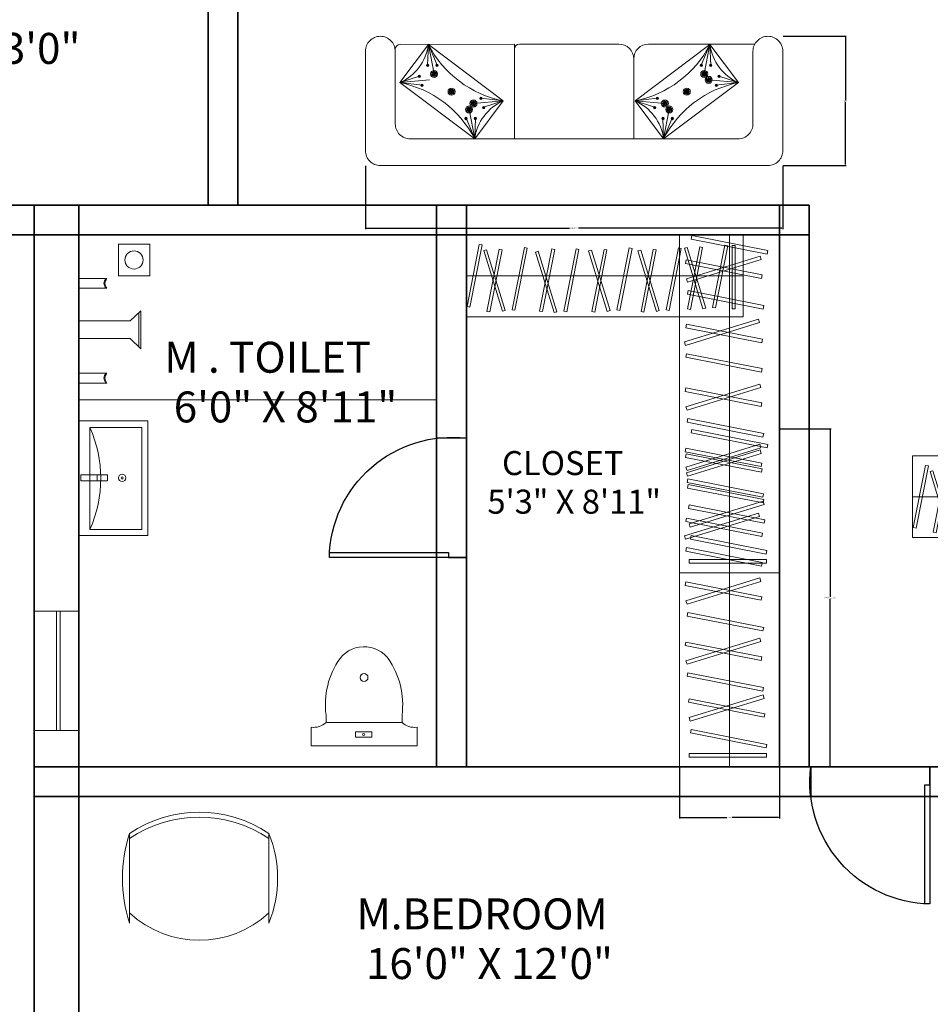
# Model space of a CAD drawing. Units: inches. Extents: x -61 to 1599, y -1316 to 257.
# Tile 18 of 204: x 76 to 259, y -1105 to -907. Entities that reach past the tile are written whole.
import ezdxf

# ---------------------------------------------------------------- set-up
doc = ezdxf.new("R2010")
doc.units = ezdxf.units.IN
doc.header["$MEASUREMENT"] = 0
doc.linetypes.add('ACAD_ISO02W100', pattern=[15, 12, -3])
for name, color, linetype, lineweight in [('A-ANNO-DIMS', 2, 'Continuous', 18), ('A-AREA-IDEN', 1, 'Continuous', 18), ('A-FLOR-CASE', 8, 'Continuous', 18), ('A-FLOR-FIXT', 8, 'Continuous', 18), ('A-WALL-JAMB', 4, 'ACAD_ISO02W100', 25), ('DOORS', 2, 'Continuous', 25), ('FURNITURE', 83, 'Continuous', 18), ('WALLS', 4, 'Continuous', 35), ('WINDOWS', 220, 'Continuous', 18)]:
    doc.layers.add(name, color=color, linetype=linetype, lineweight=lineweight)
doc.layers.add('FUR', color=83, linetype='Continuous')
doc.styles.get("Standard").update_dxf_attribs({"font": 'arial.ttf'})
doc.dimstyles.get("Standard").update_dxf_attribs({"dimtxt": 0.18, "dimasz": 0.18, "dimexe": 0.18, "dimexo": 0.0625, "dimgap": 0.09, "dimtad": 0, "dimtih": 1, "dimtoh": 1, "dimdec": 0, "dimzin": 0, "dimdsep": 46, "dimlunit": 3, "dimtxsty": 'Standard', "dimcen": 0.09, "dimadec": 0, "dimazin": 0, "dimtfac": 1, "dimtdec": 0, "dimtofl": 0, "dimtmove": 0, "dimatfit": 3, "dimfxl": 1, "dimtolj": 1, "dimtzin": 0, "dimarcsym": 0})

# ---------------------------------------------------------------- blocks, each defined once
blk = doc.blocks.new('DOOR-SWING-24')
blk.add_line((0, 0), (0, 3.6))
blk.add_lwpolyline([(0, 0), (0, -24), (1.05, -24), (1.05, 0)], close=True)
blk.add_arc((-0.44, 0.62), 24.62, 271.0259, 6.9559)
blk = doc.blocks.new('WIN-24IN')
for p, q in [((0, 4.5), (0, 9)), ((0, 9), (0, 0)), ((24, 9), (24, 0)), ((0, 5.19), (24, 5.19)), ((0, 4.5), (24, 4.5))]:
    blk.add_line(p, q)
blk = doc.blocks.new('WC-FLOOR-MOUNT')
for p, q in [((3.02, 4.69), (3.02, 6.17)), ((18.31, 4.69), (18.31, 6.17)), ((3.02, 4.69), (18.31, 4.69)), ((0, 0), (0, 3.75)), ((21.33, 0), (21.33, 3.75)), ((0, 0), (21.33, 0))]:
    blk.add_line(p, q)
blk.add_lwpolyline([(12.24, 1.73), (8.96, 1.73), (8.96, 2.81), (12.24, 2.81)], close=True)
for centre, radius in [((10.67, 13.73), 0.792), ((10.6, 2.27), 0.208)]:
    blk.add_circle(centre, radius)
for centre, radius, start, end in [((10.67, 13.73), 6.18, 27.6844, 141.4697), ((19.05, 8.26), 16.17, 144.824, 187.4232), ((2.28, 8.26), 16.17, 352.5768, 35.176), ((0.56, 7.25), 3.55, 260.8586, 313.6993), ((20.77, 7.25), 3.55, 226.3007, 279.1414)]:
    blk.add_arc(centre, radius, start, end)
blk = doc.blocks.new('LAVATORY-WALL-2')
blk.add_line((3.67, 10.96), (3.67, 12.19))
for points in [[(0, 23.07), (13.87, 23.07), (13.87, 0), (0, 0)], [(12.66, 21.73), (12.66, 1.19), (2.2, 1.19), (2.2, 21.73)], [(5.78, 12.19), (5.78, 10.96), (0.4, 10.96), (0.4, 12.19)]]:
    blk.add_lwpolyline(points, close=True)
for radius in [0.74, 0.233]:
    blk.add_circle((8.7, 11.57), radius)
blk.add_arc((-20.86, 11.46), 25.25, 335.9939, 24.0061)
blk = doc.blocks.new('SHOWER-FITTINGS-3')
for p, q in [((0, 21.03), (5.62, 21.03)), ((0, 19.05), (5.62, 19.05)), ((10.34, 12.49), (12.46, 14.54)), ((12.05, 14.15), (12.05, 7.29)), ((12.46, 14.54), (12.46, 6.9)), ((0, 12.49), (10.34, 12.49)), ((0, 8.95), (10.34, 8.95)), ((10.34, 8.95), (12.46, 6.9)), ((0, 1.97), (5.62, 1.97)), ((0, 0), (5.62, 0))]:
    blk.add_line(p, q)
blk.add_lwpolyline([(14.24, 21.57), (7.95, 21.57), (7.95, 27.94), (14.24, 27.94)], close=True)
blk.add_circle((11.09, 24.76), 1.83)
for points in [[(5.44, 21.03), (5.24, 20.71), (4.83, 20.05), (5.23, 19.39), (5.44, 19.05)], [(5.62, 21.03), (5.42, 20.71), (5.02, 20.05), (5.42, 19.39), (5.62, 19.05)], [(5.44, 1.97), (5.24, 1.65), (4.83, 1), (5.23, 0.34), (5.44, 0)], [(5.62, 1.97), (5.42, 1.65), (5.02, 1), (5.42, 0.34), (5.62, 0)]]:
    blk.add_open_spline(points, degree=3, knots=[0, 0, 0, 0, 1.043806, 2.132489, 2.132489, 2.132489, 2.132489])
blk = doc.blocks.new('BEDROOM-CHAIR')
for p, q in [((1.45, 3.47), (1.45, 21.47)), ((29.49, 3.47), (29.49, 21.47))]:
    blk.add_line(p, q)
for centre, radius, start, end in [((15.47, 0.83), 24.95, 55.8098, 124.1902), ((15.47, -0.17), 24.95, 55.8098, 124.1902), ((28.58, 12.47), 28.58, 161.6455, 198.3545), ((7.26, 12.47), 23.99, 337.9646, 22.0354), ((15.47, 20.69), 20.68, 227.332, 312.668)]:
    blk.add_arc(centre, radius, start, end)
blk = doc.blocks.new('WARDROBE-HANGING')
blk.add_line((10.05, 0), (10.05, 68))
for points in [[(20.09, 0), (0, 0), (0, 68), (20.09, 68)], [(2.48, 67.85), (17.75, 64.85), (17.61, 64.14), (2.34, 67.15)], [(1.35, 59.16), (16.22, 63.73), (16.43, 63.04), (1.56, 58.47)], [(1.32, 62.96), (16.59, 59.95), (16.45, 59.25), (1.19, 62.25)], [(1.71, 56.78), (16.98, 53.78), (16.84, 53.07), (1.57, 56.08)], [(1, 46.47), (15.87, 51.04), (16.08, 50.35), (1.21, 45.78)], [(1.39, 50.01), (16.66, 47.01), (16.52, 46.3), (1.26, 49.31)], [(1.36, 44.09), (16.63, 41.09), (16.49, 40.38), (1.23, 43.38)], [(1.28, 33.41), (16.16, 37.98), (16.37, 37.29), (1.49, 32.72)], [(1.26, 37.2), (16.53, 34.2), (16.39, 33.49), (1.12, 36.5)], [(1.65, 31.03), (16.92, 28.03), (16.78, 27.32), (1.51, 30.32)], [(1.28, 21.3), (16.15, 25.87), (16.36, 25.18), (1.49, 20.61)], [(1.26, 25.09), (16.53, 22.09), (16.39, 21.38), (1.12, 24.39)], [(1.65, 18.92), (16.91, 15.92), (16.78, 15.21), (1.51, 18.21)], [(1.93, 9.89), (16.8, 14.46), (17.01, 13.77), (2.14, 9.2)], [(1.91, 13.69), (17.17, 10.68), (17.04, 9.98), (1.77, 12.98)], [(2.29, 7.51), (17.56, 4.51), (17.42, 3.8), (2.16, 6.81)], [(17.49, 1.96), (1.93, 1.96), (1.93, 2.68), (17.49, 2.68)]]:
    blk.add_lwpolyline(points, close=True)
blk = doc.blocks.new('WARDROBE-HANGING-2')
blk.add_line((55.7, 8.23), (0, 8.23))
for points in [[(55.7, 16.46), (55.7, 0), (0, 0), (0, 16.46)], [(0.12, 2.03), (2.58, 14.54), (3.16, 14.43), (0.7, 1.92)], [(9.19, 1.4), (11.65, 13.91), (12.23, 13.8), (9.77, 1.29)], [(47.6, 1.58), (43.86, 13.76), (44.42, 13.94), (48.16, 1.75)], [(44.49, 1.56), (46.95, 14.07), (47.53, 13.95), (45.07, 1.45)], [(49.55, 1.88), (52.01, 14.39), (52.59, 14.27), (50.13, 1.77)], [(54.1, 14.33), (54.1, 1.58), (53.51, 1.58), (53.51, 14.33)], [(7.24, 1.1), (3.5, 13.29), (4.06, 13.46), (7.8, 1.28)], [(4.13, 1.08), (6.59, 13.59), (7.17, 13.48), (4.71, 0.97)], [(17.64, 0.82), (13.9, 13), (14.46, 13.18), (18.2, 0.99)], [(14.73, 1.14), (17.19, 13.65), (17.77, 13.54), (15.31, 1.03)], [(19.59, 1.12), (22.05, 13.62), (22.63, 13.51), (20.17, 1)], [(28.34, 1.05), (24.59, 13.24), (25.16, 13.41), (28.9, 1.22)], [(25.23, 1.03), (27.69, 13.54), (28.27, 13.43), (25.81, 0.92)], [(30.28, 1.35), (32.74, 13.86), (33.32, 13.75), (30.86, 1.24)], [(38.26, 1.05), (34.51, 13.23), (35.08, 13.41), (38.82, 1.22)], [(35.15, 1.03), (37.61, 13.54), (38.19, 13.42), (35.73, 0.92)], [(40.2, 1.35), (42.66, 13.86), (43.24, 13.74), (40.78, 1.23)]]:
    blk.add_lwpolyline(points, close=True)
blk = doc.blocks.new('WARDROBE-HANGING-3')
blk.add_line((10.05, 0), (10.05, 68))
blk.add_lwpolyline([(20.09, 68), (20.09, 68), (20.09, 0), (0, 0), (0, 68)])
for points in [[(2.48, 67.85), (17.75, 64.85), (17.61, 64.14), (2.34, 67.15)], [(1.35, 59.16), (16.22, 63.73), (16.43, 63.04), (1.56, 58.47)], [(1.32, 62.96), (16.59, 59.95), (16.45, 59.25), (1.19, 62.25)], [(1.71, 56.78), (16.98, 53.78), (16.84, 53.07), (1.57, 56.08)], [(1, 46.47), (15.87, 51.04), (16.08, 50.35), (1.21, 45.78)], [(1.39, 50.01), (16.66, 47.01), (16.52, 46.3), (1.26, 49.31)], [(1.36, 44.09), (16.63, 41.09), (16.49, 40.38), (1.23, 43.38)], [(1.28, 33.41), (16.16, 37.98), (16.37, 37.29), (1.49, 32.72)], [(1.26, 37.2), (16.53, 34.2), (16.39, 33.49), (1.12, 36.5)], [(1.65, 31.03), (16.92, 28.03), (16.78, 27.32), (1.51, 30.32)], [(1.28, 21.3), (16.15, 25.87), (16.36, 25.18), (1.49, 20.61)], [(1.26, 25.09), (16.53, 22.09), (16.39, 21.38), (1.12, 24.39)], [(1.65, 18.92), (16.91, 15.92), (16.78, 15.21), (1.51, 18.21)], [(1.93, 9.89), (16.8, 14.46), (17.01, 13.77), (2.14, 9.2)], [(1.91, 13.69), (17.17, 10.68), (17.04, 9.98), (1.77, 12.98)], [(2.29, 7.51), (17.56, 4.51), (17.42, 3.8), (2.16, 6.81)], [(17.49, 1.96), (1.93, 1.96), (1.93, 2.68), (17.49, 2.68)]]:
    blk.add_lwpolyline(points, close=True)
blk = doc.blocks.new('*U368')
at = {"layer": 'FUR'}
blk.add_open_spline([(0, 0.08), (-0.03, 0.05), (-0.1, -0.02), (0.08, -0.02), (0.02, -0.06), (0, -0.08)], degree=3, knots=[0, 0, 0, 0, 0.0954578, 0.1898773, 0.2470677, 0.2470677, 0.2470677, 0.2470677], dxfattribs=at)
blk = doc.blocks.new('*U369')
at = {"layer": 'FUR', "transparency": 16777216}
for p, rotation in [((222.17, -79.98), 60), ((222.18, -80.06), 120), ((222.31, -79.97), 300), ((222.25, -80.09), 180), ((222.32, -80.05), 240)]:
    blk.add_blockref('*U368', p, dxfattribs=dict(at, rotation=rotation))
blk.add_blockref('*U368', (222.24, -79.93), dxfattribs=at)
blk = doc.blocks.new('*U370')
at = {"layer": 'FUR'}
blk.add_open_spline([(0, 0.08), (-0.03, 0.05), (-0.1, -0.02), (0.08, -0.02), (0.02, -0.06), (0, -0.08)], degree=3, knots=[0, 0, 0, 0, 0.0954578, 0.1898773, 0.2470677, 0.2470677, 0.2470677, 0.2470677], dxfattribs=at)
blk = doc.blocks.new('*U371')
at = {"layer": 'FUR', "transparency": 16777216}
for p, rotation in [((222.17, -79.98), 60), ((222.18, -80.06), 120), ((222.31, -79.97), 300), ((222.25, -80.09), 180), ((222.32, -80.05), 240)]:
    blk.add_blockref('*U370', p, dxfattribs=dict(at, rotation=rotation))
blk.add_blockref('*U370', (222.24, -79.93), dxfattribs=at)
blk = doc.blocks.new('*U364')
at = {"layer": 'FUR'}
blk.add_open_spline([(0, 0.08), (-0.03, 0.05), (-0.1, -0.02), (0.08, -0.02), (0.02, -0.06), (0, -0.08)], degree=3, knots=[0, 0, 0, 0, 0.0954578, 0.1898773, 0.2470677, 0.2470677, 0.2470677, 0.2470677], dxfattribs=at)
blk = doc.blocks.new('*U365')
at = {"layer": 'FUR', "transparency": 16777216}
for p, rotation in [((222.17, -79.98), 60), ((222.18, -80.06), 120), ((222.31, -79.97), 300), ((222.25, -80.09), 180), ((222.32, -80.05), 240)]:
    blk.add_blockref('*U364', p, dxfattribs=dict(at, rotation=rotation))
blk.add_blockref('*U364', (222.24, -79.93), dxfattribs=at)
blk = doc.blocks.new('*U333')
at = {"layer": 'FUR'}
blk.add_open_spline([(0.01, 0.24), (-0.09, 0.14), (-0.29, -0.05), (0.22, -0.05), (0.07, -0.19), (0.01, -0.24)], degree=3, knots=[0, 0, 0, 0, 0.2846533, 0.5662105, 0.736751, 0.736751, 0.736751, 0.736751], dxfattribs=at)
blk = doc.blocks.new('*U334')
at = {"layer": 'FUR', "transparency": 16777216}
for p, rotation in [((662.52, -238.49), 60), ((662.53, -238.73), 120), ((662.74, -238.83), 180), ((662.93, -238.46), 300), ((662.94, -238.7), 240)]:
    blk.add_blockref('*U333', p, dxfattribs=dict(at, rotation=rotation))
blk.add_blockref('*U333', (662.72, -238.36), dxfattribs=at)
blk = doc.blocks.new('*U366')
at = {"layer": 'FUR'}
blk.add_open_spline([(0, 0.08), (-0.03, 0.05), (-0.1, -0.02), (0.08, -0.02), (0.02, -0.06), (0, -0.08)], degree=3, knots=[0, 0, 0, 0, 0.0954578, 0.1898773, 0.2470677, 0.2470677, 0.2470677, 0.2470677], dxfattribs=at)
blk = doc.blocks.new('*U367')
at = {"layer": 'FUR', "transparency": 16777216}
for p, rotation in [((222.17, -79.98), 60), ((222.18, -80.06), 120), ((222.31, -79.97), 300), ((222.25, -80.09), 180), ((222.32, -80.05), 240)]:
    blk.add_blockref('*U366', p, dxfattribs=dict(at, rotation=rotation))
blk.add_blockref('*U366', (222.24, -79.93), dxfattribs=at)
blk = doc.blocks.new('*U337')
at = {"layer": 'FUR'}
blk.add_open_spline([(0.01, 0.24), (-0.09, 0.14), (-0.29, -0.05), (0.22, -0.05), (0.07, -0.19), (0.01, -0.24)], degree=3, knots=[0, 0, 0, 0, 0.2846533, 0.5662105, 0.736751, 0.736751, 0.736751, 0.736751], dxfattribs=at)
blk = doc.blocks.new('*U338')
at = {"layer": 'FUR', "transparency": 16777216}
for p, rotation in [((662.52, -238.49), 60), ((662.53, -238.73), 120), ((662.74, -238.83), 180), ((662.93, -238.46), 300), ((662.94, -238.7), 240)]:
    blk.add_blockref('*U337', p, dxfattribs=dict(at, rotation=rotation))
blk.add_blockref('*U337', (662.72, -238.36), dxfattribs=at)
blk = doc.blocks.new('*U352')
at = {"layer": 'FUR'}
blk.add_open_spline([(0, 0.08), (-0.03, 0.05), (-0.1, -0.02), (0.08, -0.02), (0.02, -0.06), (0, -0.08)], degree=3, knots=[0, 0, 0, 0, 0.0954578, 0.1898773, 0.2470677, 0.2470677, 0.2470677, 0.2470677], dxfattribs=at)
blk = doc.blocks.new('*U353')
at = {"layer": 'FUR', "transparency": 16777216}
for p, rotation in [((222.17, -79.98), 60), ((222.18, -80.06), 120), ((222.31, -79.97), 300), ((222.25, -80.09), 180), ((222.32, -80.05), 240)]:
    blk.add_blockref('*U352', p, dxfattribs=dict(at, rotation=rotation))
blk.add_blockref('*U352', (222.24, -79.93), dxfattribs=at)
blk = doc.blocks.new('*U339')
at = {"layer": 'FUR'}
blk.add_open_spline([(0.01, 0.24), (-0.09, 0.14), (-0.29, -0.05), (0.22, -0.05), (0.07, -0.19), (0.01, -0.24)], degree=3, knots=[0, 0, 0, 0, 0.2846533, 0.5662105, 0.736751, 0.736751, 0.736751, 0.736751], dxfattribs=at)
blk = doc.blocks.new('*U351')
at = {"layer": 'FUR', "transparency": 16777216}
for p, rotation in [((662.52, -238.49), 60), ((662.53, -238.73), 120), ((662.74, -238.83), 180), ((662.93, -238.46), 300), ((662.94, -238.7), 240)]:
    blk.add_blockref('*U339', p, dxfattribs=dict(at, rotation=rotation))
blk.add_blockref('*U339', (662.72, -238.36), dxfattribs=at)
blk = doc.blocks.new('*U335')
at = {"layer": 'FUR'}
blk.add_open_spline([(0.01, 0.24), (-0.09, 0.14), (-0.29, -0.05), (0.22, -0.05), (0.07, -0.19), (0.01, -0.24)], degree=3, knots=[0, 0, 0, 0, 0.2846533, 0.5662105, 0.736751, 0.736751, 0.736751, 0.736751], dxfattribs=at)
blk = doc.blocks.new('*U336')
at = {"layer": 'FUR', "transparency": 16777216}
for p, rotation in [((662.52, -238.49), 60), ((662.53, -238.73), 120), ((662.74, -238.83), 180), ((662.93, -238.46), 300), ((662.94, -238.7), 240)]:
    blk.add_blockref('*U335', p, dxfattribs=dict(at, rotation=rotation))
blk.add_blockref('*U335', (662.72, -238.36), dxfattribs=at)
blk = doc.blocks.new('*U331')
at = {"layer": 'FUR'}
blk.add_open_spline([(0, 0.08), (-0.03, 0.05), (-0.1, -0.02), (0.08, -0.02), (0.02, -0.06), (0, -0.08)], degree=3, knots=[0, 0, 0, 0, 0.0954578, 0.1898773, 0.2470677, 0.2470677, 0.2470677, 0.2470677], dxfattribs=at)
blk = doc.blocks.new('*U332')
at = {"layer": 'FUR', "transparency": 16777216}
for p, rotation in [((222.17, -79.98), 60), ((222.18, -80.06), 120), ((222.31, -79.97), 300), ((222.25, -80.09), 180), ((222.32, -80.05), 240)]:
    blk.add_blockref('*U331', p, dxfattribs=dict(at, rotation=rotation))
blk.add_blockref('*U331', (222.24, -79.93), dxfattribs=at)
blk = doc.blocks.new('*U362')
at = {"layer": 'FUR'}
blk.add_open_spline([(0, 0.08), (-0.03, 0.05), (-0.1, -0.02), (0.08, -0.02), (0.02, -0.06), (0, -0.08)], degree=3, knots=[0, 0, 0, 0, 0.0954578, 0.1898773, 0.2470677, 0.2470677, 0.2470677, 0.2470677], dxfattribs=at)
blk = doc.blocks.new('*U363')
at = {"layer": 'FUR', "transparency": 16777216}
for p, rotation in [((222.17, -79.98), 60), ((222.18, -80.06), 120), ((222.31, -79.97), 300), ((222.25, -80.09), 180), ((222.32, -80.05), 240)]:
    blk.add_blockref('*U362', p, dxfattribs=dict(at, rotation=rotation))
blk.add_blockref('*U362', (222.24, -79.93), dxfattribs=at)
blk = doc.blocks.new('*U360')
at = {"layer": 'FUR'}
blk.add_open_spline([(0, 0.08), (-0.03, 0.05), (-0.1, -0.02), (0.08, -0.02), (0.02, -0.06), (0, -0.08)], degree=3, knots=[0, 0, 0, 0, 0.0954578, 0.1898773, 0.2470677, 0.2470677, 0.2470677, 0.2470677], dxfattribs=at)
blk = doc.blocks.new('*U361')
at = {"layer": 'FUR', "transparency": 16777216}
for p, rotation in [((222.17, -79.98), 60), ((222.18, -80.06), 120), ((222.31, -79.97), 300), ((222.25, -80.09), 180), ((222.32, -80.05), 240)]:
    blk.add_blockref('*U360', p, dxfattribs=dict(at, rotation=rotation))
blk.add_blockref('*U360', (222.24, -79.93), dxfattribs=at)
blk = doc.blocks.new('*U330')
at = {"layer": 'FUR'}
blk.add_open_spline([(0, 0.08), (-0.03, 0.05), (-0.1, -0.02), (0.08, -0.02), (0.02, -0.06), (0, -0.08)], degree=3, knots=[0, 0, 0, 0, 0.0954578, 0.1898773, 0.2470677, 0.2470677, 0.2470677, 0.2470677], dxfattribs=at)
blk = doc.blocks.new('*U343')
at = {"layer": 'FUR', "transparency": 16777216}
for p, rotation in [((222.17, -79.98), 60), ((222.18, -80.06), 120), ((222.31, -79.97), 300), ((222.25, -80.09), 180), ((222.32, -80.05), 240)]:
    blk.add_blockref('*U330', p, dxfattribs=dict(at, rotation=rotation))
blk.add_blockref('*U330', (222.24, -79.93), dxfattribs=at)
blk = doc.blocks.new('*U344')
at = {"layer": 'FUR'}
blk.add_open_spline([(0, 0.08), (-0.03, 0.05), (-0.1, -0.02), (0.08, -0.02), (0.02, -0.06), (0, -0.08)], degree=3, knots=[0, 0, 0, 0, 0.0954578, 0.1898773, 0.2470677, 0.2470677, 0.2470677, 0.2470677], dxfattribs=at)
blk = doc.blocks.new('*U345')
at = {"layer": 'FUR', "transparency": 16777216}
for p, rotation in [((222.17, -79.98), 60), ((222.18, -80.06), 120), ((222.31, -79.97), 300), ((222.25, -80.09), 180), ((222.32, -80.05), 240)]:
    blk.add_blockref('*U344', p, dxfattribs=dict(at, rotation=rotation))
blk.add_blockref('*U344', (222.24, -79.93), dxfattribs=at)
blk = doc.blocks.new('*U328')
at = {"layer": 'FUR'}
blk.add_open_spline([(0, 0.08), (-0.03, 0.05), (-0.1, -0.02), (0.08, -0.02), (0.02, -0.06), (0, -0.08)], degree=3, knots=[0, 0, 0, 0, 0.0954578, 0.1898773, 0.2470677, 0.2470677, 0.2470677, 0.2470677], dxfattribs=at)
blk = doc.blocks.new('*U329')
at = {"layer": 'FUR', "transparency": 16777216}
for p, rotation in [((222.17, -79.98), 60), ((222.18, -80.06), 120), ((222.31, -79.97), 300), ((222.25, -80.09), 180), ((222.32, -80.05), 240)]:
    blk.add_blockref('*U328', p, dxfattribs=dict(at, rotation=rotation))
blk.add_blockref('*U328', (222.24, -79.93), dxfattribs=at)
blk = doc.blocks.new('*U358')
at = {"layer": 'FUR'}
blk.add_open_spline([(0.01, 0.24), (-0.09, 0.14), (-0.29, -0.05), (0.22, -0.05), (0.07, -0.19), (0.01, -0.24)], degree=3, knots=[0, 0, 0, 0, 0.2846533, 0.5662105, 0.736751, 0.736751, 0.736751, 0.736751], dxfattribs=at)
blk = doc.blocks.new('*U359')
at = {"layer": 'FUR', "transparency": 16777216}
for p, rotation in [((662.52, -238.49), 60), ((662.53, -238.73), 120), ((662.74, -238.83), 180), ((662.93, -238.46), 300), ((662.94, -238.7), 240)]:
    blk.add_blockref('*U358', p, dxfattribs=dict(at, rotation=rotation))
blk.add_blockref('*U358', (662.72, -238.36), dxfattribs=at)
blk = doc.blocks.new('*U374')
at = {"layer": 'FUR'}
blk.add_open_spline([(0.01, 0.24), (-0.09, 0.14), (-0.29, -0.05), (0.22, -0.05), (0.07, -0.19), (0.01, -0.24)], degree=3, knots=[0, 0, 0, 0, 0.2846533, 0.5662105, 0.736751, 0.736751, 0.736751, 0.736751], dxfattribs=at)
blk = doc.blocks.new('*U325')
at = {"layer": 'FUR', "transparency": 16777216}
for p, rotation in [((662.52, -238.49), 60), ((662.53, -238.73), 120), ((662.74, -238.83), 180), ((662.93, -238.46), 300), ((662.94, -238.7), 240)]:
    blk.add_blockref('*U374', p, dxfattribs=dict(at, rotation=rotation))
blk.add_blockref('*U374', (662.72, -238.36), dxfattribs=at)
blk = doc.blocks.new('*U326')
at = {"layer": 'FUR'}
blk.add_open_spline([(0, 0.08), (-0.03, 0.05), (-0.1, -0.02), (0.08, -0.02), (0.02, -0.06), (0, -0.08)], degree=3, knots=[0, 0, 0, 0, 0.0954578, 0.1898773, 0.2470677, 0.2470677, 0.2470677, 0.2470677], dxfattribs=at)
blk = doc.blocks.new('*U327')
at = {"layer": 'FUR', "transparency": 16777216}
for p, rotation in [((222.17, -79.98), 60), ((222.18, -80.06), 120), ((222.31, -79.97), 300), ((222.25, -80.09), 180), ((222.32, -80.05), 240)]:
    blk.add_blockref('*U326', p, dxfattribs=dict(at, rotation=rotation))
blk.add_blockref('*U326', (222.24, -79.93), dxfattribs=at)
blk = doc.blocks.new('*U372')
at = {"layer": 'FUR'}
blk.add_open_spline([(0.01, 0.24), (-0.09, 0.14), (-0.29, -0.05), (0.22, -0.05), (0.07, -0.19), (0.01, -0.24)], degree=3, knots=[0, 0, 0, 0, 0.2846533, 0.5662105, 0.736751, 0.736751, 0.736751, 0.736751], dxfattribs=at)
blk = doc.blocks.new('*U373')
at = {"layer": 'FUR', "transparency": 16777216}
for p, rotation in [((662.52, -238.49), 60), ((662.53, -238.73), 120), ((662.74, -238.83), 180), ((662.93, -238.46), 300), ((662.94, -238.7), 240)]:
    blk.add_blockref('*U372', p, dxfattribs=dict(at, rotation=rotation))
blk.add_blockref('*U372', (662.72, -238.36), dxfattribs=at)
blk = doc.blocks.new('*U348')
at = {"layer": 'FUR'}
blk.add_open_spline([(0, 0.08), (-0.03, 0.05), (-0.1, -0.02), (0.08, -0.02), (0.02, -0.06), (0, -0.08)], degree=3, knots=[0, 0, 0, 0, 0.0954578, 0.1898773, 0.2470677, 0.2470677, 0.2470677, 0.2470677], dxfattribs=at)
blk = doc.blocks.new('*U349')
at = {"layer": 'FUR', "transparency": 16777216}
for p, rotation in [((222.17, -79.98), 60), ((222.18, -80.06), 120), ((222.31, -79.97), 300), ((222.25, -80.09), 180), ((222.32, -80.05), 240)]:
    blk.add_blockref('*U348', p, dxfattribs=dict(at, rotation=rotation))
blk.add_blockref('*U348', (222.24, -79.93), dxfattribs=at)
blk = doc.blocks.new('*U356')
at = {"layer": 'FUR'}
blk.add_open_spline([(0.01, 0.24), (-0.09, 0.14), (-0.29, -0.05), (0.22, -0.05), (0.07, -0.19), (0.01, -0.24)], degree=3, knots=[0, 0, 0, 0, 0.2846533, 0.5662105, 0.736751, 0.736751, 0.736751, 0.736751], dxfattribs=at)
blk = doc.blocks.new('*U357')
at = {"layer": 'FUR', "transparency": 16777216}
for p, rotation in [((662.52, -238.49), 60), ((662.53, -238.73), 120), ((662.74, -238.83), 180), ((662.93, -238.46), 300), ((662.94, -238.7), 240)]:
    blk.add_blockref('*U356', p, dxfattribs=dict(at, rotation=rotation))
blk.add_blockref('*U356', (662.72, -238.36), dxfattribs=at)
blk = doc.blocks.new('*U340')
at = {"layer": 'FUR'}
blk.add_open_spline([(0.01, 0.24), (-0.09, 0.14), (-0.29, -0.05), (0.22, -0.05), (0.07, -0.19), (0.01, -0.24)], degree=3, knots=[0, 0, 0, 0, 0.2846533, 0.5662105, 0.736751, 0.736751, 0.736751, 0.736751], dxfattribs=at)
blk = doc.blocks.new('*U341')
at = {"layer": 'FUR', "transparency": 16777216}
for p, rotation in [((662.52, -238.49), 60), ((662.53, -238.73), 120), ((662.74, -238.83), 180), ((662.93, -238.46), 300), ((662.94, -238.7), 240)]:
    blk.add_blockref('*U340', p, dxfattribs=dict(at, rotation=rotation))
blk.add_blockref('*U340', (662.72, -238.36), dxfattribs=at)
blk = doc.blocks.new('*U346')
at = {"layer": 'FUR'}
blk.add_open_spline([(0, 0.08), (-0.03, 0.05), (-0.1, -0.02), (0.08, -0.02), (0.02, -0.06), (0, -0.08)], degree=3, knots=[0, 0, 0, 0, 0.0954578, 0.1898773, 0.2470677, 0.2470677, 0.2470677, 0.2470677], dxfattribs=at)
blk = doc.blocks.new('*U347')
at = {"layer": 'FUR', "transparency": 16777216}
for p, rotation in [((222.17, -79.98), 60), ((222.18, -80.06), 120), ((222.31, -79.97), 300), ((222.25, -80.09), 180), ((222.32, -80.05), 240)]:
    blk.add_blockref('*U346', p, dxfattribs=dict(at, rotation=rotation))
blk.add_blockref('*U346', (222.24, -79.93), dxfattribs=at)
blk = doc.blocks.new('*U354')
at = {"layer": 'FUR'}
blk.add_open_spline([(0, 0.08), (-0.03, 0.05), (-0.1, -0.02), (0.08, -0.02), (0.02, -0.06), (0, -0.08)], degree=3, knots=[0, 0, 0, 0, 0.0954578, 0.1898773, 0.2470677, 0.2470677, 0.2470677, 0.2470677], dxfattribs=at)
blk = doc.blocks.new('*U355')
at = {"layer": 'FUR', "transparency": 16777216}
for p, rotation in [((222.17, -79.98), 60), ((222.18, -80.06), 120), ((222.31, -79.97), 300), ((222.25, -80.09), 180), ((222.32, -80.05), 240)]:
    blk.add_blockref('*U354', p, dxfattribs=dict(at, rotation=rotation))
blk.add_blockref('*U354', (222.24, -79.93), dxfattribs=at)
blk = doc.blocks.new('*U350')
at = {"layer": 'FUR'}
blk.add_open_spline([(0, 0.08), (-0.03, 0.05), (-0.1, -0.02), (0.08, -0.02), (0.02, -0.06), (0, -0.08)], degree=3, knots=[0, 0, 0, 0, 0.0954578, 0.1898773, 0.2470677, 0.2470677, 0.2470677, 0.2470677], dxfattribs=at)
blk = doc.blocks.new('*U342')
at = {"layer": 'FUR', "transparency": 16777216}
for p, rotation in [((222.17, -79.98), 60), ((222.18, -80.06), 120), ((222.31, -79.97), 300), ((222.25, -80.09), 180), ((222.32, -80.05), 240)]:
    blk.add_blockref('*U350', p, dxfattribs=dict(at, rotation=rotation))
blk.add_blockref('*U350', (222.24, -79.93), dxfattribs=at)
blk = doc.blocks.new('SOFA-THREE-SEAT-ALT')
for p, q in [((30, 24.44), (7, 24.38)), ((12.66, 24.33), (12.51, 20.19)), ((12.66, 24.33), (13.81, 18.42)), ((12.66, 24.33), (14.41, 20.19)), ((30, 23.44), (30, 24.44)), ((51, 24.44), (31, 24.44)), ((78.37, 24.44), (57, 24.44)), ((69.34, 24.33), (67.59, 20.19)), ((69.34, 24.33), (68.19, 18.42)), ((69.34, 24.33), (69.49, 20.19)), ((6, 23), (6, 23.38)), ((30, 23.44), (30, 5.38)), ((12.49, 20.14), (12.49, 20.3)), ((12.49, 20.14), (12.49, 19.98)), ((14.39, 20.14), (14.39, 20.3)), ((14.39, 20.14), (14.39, 19.98)), ((54, 21.44), (54, 5.38)), ((54, 21.44), (54, 21.44)), ((67.6, 20.14), (67.6, 20.3)), ((67.6, 20.14), (67.6, 19.98)), ((69.51, 20.14), (69.51, 20.3)), ((69.51, 20.14), (69.51, 19.98)), ((6.93, 16.69), (10.86, 17.99)), ((10.84, 17.94), (10.84, 18.1)), ((10.84, 17.94), (10.84, 17.78)), ((13.81, 18.42), (13.81, 18.9)), ((13.81, 18.42), (13.81, 17.95)), ((68.19, 18.42), (68.19, 18.9)), ((68.19, 18.42), (68.19, 17.95)), ((75.07, 16.69), (71.14, 17.99)), ((71.16, 17.94), (71.16, 18.1)), ((71.16, 17.94), (71.16, 17.78)), ((6.93, 16.69), (12.92, 17.24)), ((6.93, 16.69), (11.39, 16.16)), ((11.37, 16.11), (11.37, 16.27)), ((11.37, 16.11), (11.37, 15.95)), ((69.08, 17.24), (69.08, 17.72)), ((75.07, 16.69), (69.08, 17.24)), ((69.08, 17.24), (69.08, 16.77)), ((75.07, 16.69), (70.61, 16.16)), ((70.63, 16.11), (70.63, 16.27)), ((70.63, 16.11), (70.63, 15.95)), ((17.33, 14.86), (17.33, 15.33)), ((17.33, 14.86), (17.33, 14.38)), ((64.67, 14.86), (64.67, 15.33)), ((64.67, 14.86), (64.67, 14.38)), ((27.73, 13.03), (21.73, 12.47)), ((21.73, 12.47), (21.73, 12.95)), ((21.73, 12.47), (21.73, 12)), ((23.24, 13.5), (23.24, 13.66)), ((23.24, 13.5), (23.24, 13.34)), ((27.73, 13.03), (23.26, 13.55)), ((27.73, 13.03), (23.79, 11.72)), ((54.27, 13.03), (58.74, 13.55)), ((54.27, 13.03), (60.26, 12.47)), ((54.27, 13.03), (58.2, 11.72)), ((58.76, 13.5), (58.76, 13.66)), ((58.76, 13.5), (58.76, 13.34)), ((60.26, 12.47), (60.26, 12.95)), ((60.26, 12.47), (60.26, 12)), ((20.85, 11.29), (20.85, 11.77)), ((21.99, 5.38), (20.85, 11.29)), ((20.85, 11.29), (20.85, 10.82)), ((23.78, 11.67), (23.78, 11.83)), ((23.78, 11.67), (23.78, 11.51)), ((58.22, 11.67), (58.22, 11.83)), ((58.22, 11.67), (58.22, 11.51)), ((60.01, 5.38), (61.15, 11.29)), ((61.15, 11.29), (61.15, 11.77)), ((61.15, 11.29), (61.15, 10.82)), ((20.22, 9.47), (20.22, 9.63)), ((20.22, 9.47), (20.22, 9.31)), ((21.99, 5.38), (20.24, 9.52)), ((21.99, 5.38), (22.14, 9.52)), ((22.13, 9.47), (22.13, 9.63)), ((22.13, 9.47), (22.13, 9.31)), ((60.01, 5.38), (59.85, 9.52)), ((59.87, 9.47), (59.87, 9.63)), ((59.87, 9.47), (59.87, 9.31)), ((60.01, 5.38), (61.76, 9.52)), ((61.78, 9.47), (61.78, 9.63)), ((61.78, 9.47), (61.78, 9.31))]:
    blk.add_line(p, q)
blk.add_lwpolyline([(78, 8.38), (78, 23, -0.414214), (81, 26), (81, 26, -0.414214), (84, 23), (84, 3, -0.414214), (81, 0), (3, 0, -0.414214), (0, 3), (0, 23, -0.414214), (3, 26), (3, 26, -0.414214), (6, 23), (6, 8.38, 0.414214), (9, 5.38), (75, 5.38, 0.414214)], format="xyb", close=True)
for points in [[(27.73, 13.03), (12.66, 24.33), (6.93, 16.69), (21.99, 5.38)], [(54.27, 13.03), (69.34, 24.33), (75.07, 16.69), (60.01, 5.38)]]:
    blk.add_lwpolyline(points, close=True)
for centre, radius in [((12.49, 20.14), 0.238), ((12.49, 20.14), 0.16), ((14.39, 20.14), 0.238), ((14.39, 20.14), 0.16), ((67.6, 20.14), 0.238), ((67.6, 20.14), 0.16), ((69.51, 20.14), 0.238), ((69.51, 20.14), 0.16), ((10.84, 17.94), 0.238), ((10.84, 17.94), 0.16), ((13.81, 18.42), 0.71), ((13.81, 18.42), 0.476), ((68.19, 18.42), 0.71), ((68.19, 18.42), 0.476), ((69.08, 17.24), 0.71), ((71.16, 17.94), 0.238), ((71.16, 17.94), 0.16), ((11.37, 16.11), 0.238), ((11.37, 16.11), 0.16), ((69.08, 17.24), 0.476), ((70.63, 16.11), 0.238), ((70.63, 16.11), 0.16), ((17.33, 14.86), 0.71), ((17.33, 14.86), 0.476), ((64.67, 14.86), 0.71), ((64.67, 14.86), 0.476), ((20.85, 11.29), 0.71), ((21.73, 12.47), 0.71), ((21.73, 12.47), 0.476), ((23.24, 13.5), 0.238), ((23.24, 13.5), 0.16), ((23.78, 11.67), 0.238), ((58.22, 11.67), 0.238), ((58.76, 13.5), 0.238), ((58.76, 13.5), 0.16), ((60.26, 12.47), 0.71), ((60.26, 12.47), 0.476), ((61.15, 11.29), 0.71), ((20.85, 11.29), 0.476), ((23.78, 11.67), 0.16), ((58.22, 11.67), 0.16), ((61.15, 11.29), 0.476), ((20.22, 9.47), 0.238), ((20.22, 9.47), 0.16), ((22.13, 9.47), 0.238), ((22.13, 9.47), 0.16), ((59.87, 9.47), 0.238), ((59.87, 9.47), 0.16), ((61.78, 9.47), 0.238), ((61.78, 9.47), 0.16)]:
    blk.add_circle(centre, radius)
for centre, radius, start, end in [((7, 23.38), 1, 90.1542, 180.1542), ((2.94, 25.66), 9.82, 293.9742, 352.253), ((31.95, 34.34), 21.73, 207.4316, 258.7956), ((31, 23.44), 1, 90, 180), ((51, 21.44), 3, 360, 90), ((57, 21.44), 3, 90, 180), ((50.05, 34.34), 21.73, 281.2044, 332.5684), ((79.06, 25.66), 9.82, 187.747, 246.0258), ((2.7, -4.63), 21.73, 27.4316, 78.7956), ((79.3, -4.63), 21.73, 101.2044, 152.5684), ((31.72, 4.06), 9.82, 113.9742, 172.253), ((50.28, 4.06), 9.82, 7.747, 66.0258)]:
    blk.add_arc(centre, radius, start, end)
at = {"xscale": -1, "rotation": 180}
for name, p in [('*U365', (-209.75, -59.87)), ('*U367', (-207.85, -59.87)), ('*U369', (-211.41, -62.07)), ('*U334', (-648.93, -220.17)), ('*U371', (-210.87, -63.9)), ('*U338', (-645.4, -223.74)), ('*U336', (-641, -226.12)), ('*U363', (-199, -66.51)), ('*U351', (-641.88, -227.3)), ('*U361', (-198.47, -68.34)), ('*U353', (-202.02, -70.54)), ('*U332', (-200.12, -70.54))]:
    blk.add_blockref(name, p, dxfattribs=at)
at = {"rotation": 180}
for name, p in [('*U349', (289.85, -59.87)), ('*U347', (291.75, -59.87)), ('*U357', (730.92, -220.17)), ('*U342', (293.4, -62.07)), ('*U341', (731.81, -221.35)), ('*U355', (292.87, -63.9)), ('*U373', (727.4, -223.74)), ('*U345', (281, -66.51)), ('*U359', (722.99, -226.12)), ('*U343', (280.47, -68.34)), ('*U325', (723.88, -227.3)), ('*U329', (282.12, -70.54)), ('*U327', (284.02, -70.54))]:
    blk.add_blockref(name, p, dxfattribs=at)
blk = doc.blocks.new('*D668')
at = {"layer": 'A-ANNO-DIMS', "color": 0, "lineweight": -2, "transparency": 16777216}
for p, q in [((228.77, -988.94), (239.08, -988.94)), ((238.9, -989.12), (238.9, -1022.76)), ((238.9, -1056.76), (238.9, -1023.13)), ((228.77, -1056.94), (239.08, -1056.94))]:
    blk.add_line(p, q, dxfattribs=at)
at = {"layer": 'A-ANNO-DIMS', "color": 0, "transparency": 16777216}
for points in [[(238.87, -989.12), (238.93, -989.12), (238.9, -988.94)], [(238.87, -1056.76), (238.93, -1056.76), (238.9, -1056.94)]]:
    blk.add_solid(points, dxfattribs=at)
at = {"layer": 'DEFPOINTS', "color": 0, "transparency": 16777216}
for p in [(228.7, -988.94), (238.9, -988.94), (228.7, -1056.94)]:
    blk.add_point(p, dxfattribs=at)
at = {"layer": 'A-ANNO-DIMS', "color": 0, "transparency": 16777216, "insert": (238.9, -1022.94), "char_height": 0.18, "attachment_point": 5}
blk.add_mtext('\\A1;WARDROBE 68 TYP.', dxfattribs=at)
blk = doc.blocks.new('*D669')
at = {"layer": 'A-ANNO-DIMS', "color": 0, "lineweight": -2, "transparency": 16777216}
for p, q in [((208.61, -1057.01), (208.61, -1067.32)), ((228.7, -1057.01), (228.7, -1067.32)), ((208.79, -1067.14), (218.13, -1067.14)), ((228.52, -1067.14), (219.19, -1067.14))]:
    blk.add_line(p, q, dxfattribs=at)
at = {"layer": 'A-ANNO-DIMS', "color": 0, "transparency": 16777216}
for points in [[(208.79, -1067.11), (208.79, -1067.17), (208.61, -1067.14)], [(228.52, -1067.11), (228.52, -1067.17), (228.7, -1067.14)]]:
    blk.add_solid(points, dxfattribs=at)
at = {"layer": 'DEFPOINTS', "color": 0, "transparency": 16777216}
for p in [(208.61, -1056.94), (228.7, -1056.94), (228.7, -1067.14)]:
    blk.add_point(p, dxfattribs=at)
at = {"layer": 'A-ANNO-DIMS', "color": 0, "transparency": 16777216, "insert": (218.66, -1067.14), "char_height": 0.18, "attachment_point": 5}
blk.add_mtext('\\A1;20 TYP.', dxfattribs=at)
blk = doc.blocks.new('*D682')
at = {"layer": 'A-ANNO-DIMS', "color": 0, "lineweight": -2, "transparency": 16777216}
for p, q in [((145.37, -936.06), (145.37, -948.78)), ((229.37, -936.06), (229.37, -948.78)), ((145.55, -948.6), (186.47, -948.6)), ((229.19, -948.6), (188.28, -948.6))]:
    blk.add_line(p, q, dxfattribs=at)
at = {"layer": 'A-ANNO-DIMS', "color": 0, "transparency": 16777216}
for points in [[(145.55, -948.57), (145.55, -948.63), (145.37, -948.6)], [(229.19, -948.57), (229.19, -948.63), (229.37, -948.6)]]:
    blk.add_solid(points, dxfattribs=at)
at = {"layer": 'DEFPOINTS', "color": 0, "transparency": 16777216}
for p in [(145.37, -936), (229.37, -936), (229.37, -948.6)]:
    blk.add_point(p, dxfattribs=at)
at = {"layer": 'A-ANNO-DIMS', "color": 0, "transparency": 16777216, "insert": (187.37, -948.6), "char_height": 0.18, "attachment_point": 5}
blk.add_mtext('\\A1;SOFA 84 TYP.', dxfattribs=at)
blk = doc.blocks.new('*D683')
at = {"layer": 'A-ANNO-DIMS', "color": 0, "lineweight": -2, "transparency": 16777216}
for p, q in [((229.44, -910), (242.15, -910)), ((241.97, -910.18), (241.97, -922.82)), ((241.97, -935.82), (241.97, -923.18)), ((229.44, -936), (242.15, -936))]:
    blk.add_line(p, q, dxfattribs=at)
at = {"layer": 'A-ANNO-DIMS', "color": 0, "transparency": 16777216}
for points in [[(241.94, -910.18), (242, -910.18), (241.97, -910)], [(241.94, -935.82), (242, -935.82), (241.97, -936)]]:
    blk.add_solid(points, dxfattribs=at)
at = {"layer": 'DEFPOINTS', "color": 0, "transparency": 16777216}
for p in [(229.37, -910), (241.97, -910), (229.37, -936)]:
    blk.add_point(p, dxfattribs=at)
at = {"layer": 'A-ANNO-DIMS', "color": 0, "transparency": 16777216, "insert": (241.97, -923), "char_height": 0.18, "attachment_point": 5}
blk.add_mtext('\\A1;26 TYP.', dxfattribs=at)
blk = doc.blocks.new('*D687')
at = {"layer": 'A-ANNO-DIMS', "color": 0, "lineweight": -2, "transparency": 16777216}
for p, q in [((289.42, 181.68), (-61.08, 181.68)), ((-60.9, 181.5), (-60.9, -528.95)), ((-60.9, -1239.76), (-60.9, -529.32)), ((319.64, -1239.94), (-61.08, -1239.94))]:
    blk.add_line(p, q, dxfattribs=at)
at = {"layer": 'A-ANNO-DIMS', "color": 0, "transparency": 16777216}
for points in [[(-60.93, 181.5), (-60.87, 181.5), (-60.9, 181.68)], [(-60.93, -1239.76), (-60.87, -1239.76), (-60.9, -1239.94)]]:
    blk.add_solid(points, dxfattribs=at)
at = {"layer": 'DEFPOINTS', "color": 0, "transparency": 16777216}
for p in [(289.48, 181.68), (-60.9, -1239.94), (319.7, -1239.94)]:
    blk.add_point(p, dxfattribs=at)
at = {"layer": 'A-ANNO-DIMS', "color": 0, "transparency": 16777216, "insert": (-60.9, -529.13), "char_height": 0.18, "attachment_point": 5}
blk.add_mtext('\\A1;1421.6', dxfattribs=at)
blk = doc.blocks.new('*D696')
at = {"layer": 'A-ANNO-DIMS', "color": 0, "lineweight": -2, "transparency": 16777216}
for p, q in [((690.64, -873.17), (-61.08, -873.17)), ((-60.9, -873.35), (-60.9, -1025.8)), ((-60.9, -1178.61), (-60.9, -1026.16)), ((690.64, -1178.79), (-61.08, -1178.79))]:
    blk.add_line(p, q, dxfattribs=at)
at = {"layer": 'A-ANNO-DIMS', "color": 0, "transparency": 16777216}
for points in [[(-60.93, -873.35), (-60.87, -873.35), (-60.9, -873.17)], [(-60.93, -1178.61), (-60.87, -1178.61), (-60.9, -1178.79)]]:
    blk.add_solid(points, dxfattribs=at)
at = {"layer": 'DEFPOINTS', "color": 0, "transparency": 16777216}
for p in [(-60.9, -873.17), (690.7, -873.17), (690.7, -1178.79)]:
    blk.add_point(p, dxfattribs=at)
at = {"layer": 'A-ANNO-DIMS', "color": 0, "transparency": 16777216, "insert": (-60.9, -1025.98), "char_height": 0.18, "attachment_point": 5}
blk.add_mtext('\\A1;305.6', dxfattribs=at)

msp = doc.modelspace()

# ---------------------------------------------------------------- linework, layer by layer
at = {"layer": 'A-FLOR-FIXT'}
msp.add_line((87.7028, -983.1308), (159.7028, -983.1308), dxfattribs=at)
at = {"layer": 'A-WALL-JAMB'}
for p, q in [((165.7028, -990.8586), (159.7028, -990.863)), ((165.7028, -1014.8586), (159.7028, -1014.8586)), ((234.999, -1056.9446), (234.999, -1062.9446)), ((258.999, -1056.9446), (258.999, -1062.9446))]:
    msp.add_line(p, q, dxfattribs=at)
at = {"layer": 'WALLS'}
for p, q in [((113.7028, -943.9446), (113.7028, -787.9446)), ((119.7028, -943.9446), (119.7028, -787.9446)), ((14.7028, -943.9446), (234.7028, -943.9446)), ((78.7028, -943.9446), (78.7028, -1215.9446)), ((87.7028, -943.9446), (87.7028, -949.9446)), ((159.7028, -1056.9446), (159.7028, -943.9446)), ((165.7028, -1056.9446), (165.7028, -943.9446)), ((228.7028, -1056.9446), (228.7028, -943.9446)), ((234.7028, -1056.9446), (234.7028, -943.9446)), ((14.7028, -949.9446), (234.7028, -949.9446)), ((87.7028, -1056.9446), (87.7028, -949.9446)), ((78.7028, -1056.9446), (237.7028, -1056.9446)), ((87.7028, -1056.9446), (87.7028, -1215.9446)), ((237.7028, -1056.9446), (325.7028, -1056.9446)), ((78.7028, -1062.9446), (237.7028, -1062.9446)), ((237.7028, -1062.9446), (325.7028, -1062.9446))]:
    msp.add_line(p, q, dxfattribs=at)

# ---------------------------------------------------------------- block references
at = {"layer": 'A-FLOR-CASE'}
for name, p in [('WARDROBE-HANGING-2', (165.703, -966.4047)), ('WARDROBE-HANGING', (208.609, -1017.9447)), ('WARDROBE-HANGING-3', (208.609, -1056.9447)), ('WARDROBE-HANGING-2', (255.5089, -1010.847))]:
    msp.add_blockref(name, p, dxfattribs=at)
at = {"layer": 'A-FLOR-FIXT'}
for name, p in [('SHOWER-FITTINGS-3', (87.703, -979.7457)), ('LAVATORY-WALL-2', (87.703, -1010.4057)), ('WC-FLOOR-MOUNT', (134.4199, -1052.7142))]:
    msp.add_blockref(name, p, dxfattribs=at)
at = {"layer": 'DOORS', "extrusion": (0, 0, -1), "zscale": -1, "rotation": 89.99999999999973}
msp.add_blockref('DOOR-SWING-24', (-162.1028, -1014.8586), dxfattribs=at)
at = {"layer": 'DOORS', "extrusion": (0, 0, -1), "zscale": -1}
msp.add_blockref('DOOR-SWING-24', (-258.999, -1060.5446), dxfattribs=at)
at = {"layer": 'FURNITURE'}
for name, p in [('SOFA-THREE-SEAT-ALT', (145.375, -936.001)), ('BEDROOM-CHAIR', (96.4434, -1091.8396))]:
    msp.add_blockref(name, p, dxfattribs=at)
at = {"layer": 'WINDOWS', "rotation": 269.9999999999999}
msp.add_blockref('WIN-24IN', (78.7027, -1025.615), dxfattribs=at)

# ---------------------------------------------------------------- texts
at = {"layer": 'A-AREA-IDEN'}
for s, height, p in [('7\'6" X 13\'0"', 6.223643, (43.0043, -915.5424)), (' M . TOILET', 6.223643, (102.978, -977.6724)), ('  6\'0" X 8\'11"', 6.223643, (102.978, -987.6701)), ('  CLOSET', 4.8321, (169.9149, -998.2674)), ('5\'3" X 8\'11"', 4.832098, (169.9149, -1006.0297)), ('M.BEDROOM ', 6.22364, (143.5758, -1089.6444)), (' 16\'0" X 12\'0"', 6.223643, (143.5758, -1099.6421))]:
    msp.add_text(s, height=height, dxfattribs=at).set_placement(p)

# ---------------------------------------------------------------- dimensions: what is measured, and where the dimension line sits
at = {"layer": 'A-ANNO-DIMS'}
for base, p1, p2, picture, middle in [((-60.8972, -1239.9446), (289.4807, 181.6771), (319.7028, -1239.9446), '*D687', (-60.8972, -529.1337)), ((-60.8972, -873.169), (690.7028, -1178.7933), (690.7028, -873.169), '*D696', (-60.8972, -1025.9812))]:
    dim = msp.add_linear_dim(base=base, p1=p1, p2=p2, angle=90, dimstyle='Standard', override={"dimdec": 1, "dimlfac": 1, "dimrnd": 0, "dimzin": 0, "dimdsep": 46, "dimlunit": 2}, dxfattribs=at)
    dim.commit()
    dim.dimension.update_dxf_attribs({"geometry": picture, "text_midpoint": middle})
for base, p1, p2, text, picture, middle in [((241.9746, -910.0009), (229.3746, -936.0009), (229.3746, -910.0009), '<> TYP.', '*D683', (241.9746, -923.0009)), ((238.9028, -988.9446), (228.7028, -1056.9446), (228.7028, -988.9446), 'WARDROBE <> TYP.', '*D668', (238.9028, -1022.9446))]:
    dim = msp.add_linear_dim(base=base, p1=p1, p2=p2, angle=90, text=text, dimstyle='Standard', override={"dimdec": 0, "dimlfac": 1, "dimrnd": 0, "dimzin": 0, "dimdsep": 46, "dimlunit": 2}, dxfattribs=at)
    dim.commit()
    dim.dimension.update_dxf_attribs({"geometry": picture, "text_midpoint": middle})
for base, p1, p2, text, picture, middle in [((229.3746, -948.6009), (145.3746, -936.0009), (229.3746, -936.0009), 'SOFA <> TYP.', '*D682', (187.3746, -948.6009)), ((228.7028, -1067.1446), (208.6092, -1056.9446), (228.7028, -1056.9446), '<> TYP.', '*D669', (218.656, -1067.1446))]:
    dim = msp.add_linear_dim(base=base, p1=p1, p2=p2, text=text, dimstyle='Standard', override={"dimdec": 0, "dimlfac": 1, "dimrnd": 0, "dimzin": 0, "dimdsep": 46, "dimlunit": 2}, dxfattribs=at)
    dim.commit()
    dim.dimension.update_dxf_attribs({"geometry": picture, "text_midpoint": middle})

doc.saveas('drawing.dxf')
